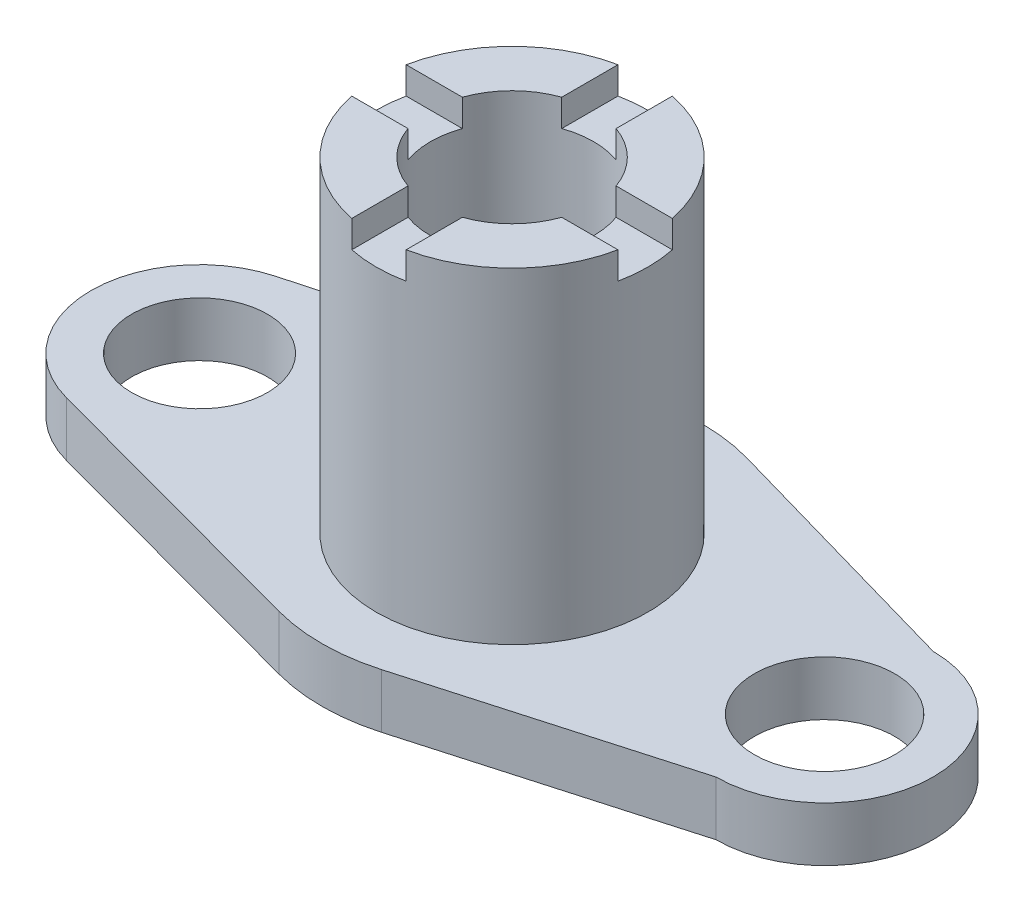
ISO-10303-21;
HEADER;
FILE_DESCRIPTION(('STEP AP214'),'2;1');
FILE_NAME('part.step','',(''),(''),'','','');
FILE_SCHEMA(('AUTOMOTIVE_DESIGN { 1 0 10303 214 1 1 1 1 }'));
ENDSEC;
DATA;
#1=APPLICATION_CONTEXT('core data for automotive mechanical design processes');
#2=APPLICATION_PROTOCOL_DEFINITION('international standard','automotive_design',2000,#1);
#3=PRODUCT_CONTEXT('',#1,'mechanical');
#4=PRODUCT('Part','Part','',(#3));
#5=PRODUCT_RELATED_PRODUCT_CATEGORY('part','',(#4));
#6=PRODUCT_DEFINITION_FORMATION('','',#4);
#7=PRODUCT_DEFINITION_CONTEXT('part definition',#1,'design');
#8=PRODUCT_DEFINITION('design','',#6,#7);
#9=PRODUCT_DEFINITION_SHAPE('','',#8);
#10=(LENGTH_UNIT() NAMED_UNIT(*) SI_UNIT(.MILLI.,.METRE.));
#11=(NAMED_UNIT(*) PLANE_ANGLE_UNIT() SI_UNIT($,.RADIAN.));
#12=(NAMED_UNIT(*) SI_UNIT($,.STERADIAN.) SOLID_ANGLE_UNIT());
#13=UNCERTAINTY_MEASURE_WITH_UNIT(LENGTH_MEASURE(1.E-05),#10,'distance_accuracy_value','');
#14=(GEOMETRIC_REPRESENTATION_CONTEXT(3) GLOBAL_UNCERTAINTY_ASSIGNED_CONTEXT((#13)) GLOBAL_UNIT_ASSIGNED_CONTEXT((#10,
#11,#12)) REPRESENTATION_CONTEXT('',''));
#15=CARTESIAN_POINT('',(0.,0.,0.));
#16=DIRECTION('',(0.,0.,1.));
#17=DIRECTION('',(1.,0.,0.));
#18=AXIS2_PLACEMENT_3D('',#15,#16,#17);
#19=CARTESIAN_POINT('',(0.,65.,0.));
#20=DIRECTION('',(0.,1.,0.));
#21=DIRECTION('',(0.,0.,1.));
#22=AXIS2_PLACEMENT_3D('',#19,#20,#21);
#23=PLANE('',#22);
#24=DIRECTION('',(0.,0.,-1.));
#25=VECTOR('',#24,1.);
#26=CARTESIAN_POINT('',(5.,65.,-25.0621356237309));
#27=LINE('',#26,#25);
#28=CARTESIAN_POINT('',(5.,65.,-14.1421356237309));
#29=VERTEX_POINT('',#28);
#30=CARTESIAN_POINT('',(5.,65.,-24.4948974278318));
#31=VERTEX_POINT('',#30);
#32=EDGE_CURVE('E249',#29,#31,#27,.T.);
#33=ORIENTED_EDGE('',*,*,#32,.F.);
#34=CARTESIAN_POINT('',(0.,65.,0.));
#35=DIRECTION('',(0.,1.,0.));
#36=DIRECTION('',(0.,0.,1.));
#37=AXIS2_PLACEMENT_3D('',#34,#35,#36);
#38=CIRCLE('',#37,15.);
#39=CARTESIAN_POINT('',(14.142135623731,65.,-4.99999999999995));
#40=VERTEX_POINT('',#39);
#41=EDGE_CURVE('E228',#40,#29,#38,.T.);
#42=ORIENTED_EDGE('',*,*,#41,.F.);
#43=DIRECTION('',(-1.,0.,0.));
#44=VECTOR('',#43,1.);
#45=CARTESIAN_POINT('',(25.062135623731,65.,-4.99999999999991));
#46=LINE('',#45,#44);
#47=CARTESIAN_POINT('',(24.4948974278318,65.,-4.99999999999991));
#48=VERTEX_POINT('',#47);
#49=EDGE_CURVE('E243',#48,#40,#46,.T.);
#50=ORIENTED_EDGE('',*,*,#49,.F.);
#51=CARTESIAN_POINT('',(0.,65.,0.));
#52=DIRECTION('',(0.,1.,0.));
#53=DIRECTION('',(0.,0.,1.));
#54=AXIS2_PLACEMENT_3D('',#51,#52,#53);
#55=CIRCLE('',#54,25.);
#56=EDGE_CURVE('E320',#48,#31,#55,.T.);
#57=ORIENTED_EDGE('',*,*,#56,.T.);
#58=EDGE_LOOP('',(#33,#42,#50,#57));
#59=FACE_BOUND('',#58,.T.);
#60=ADVANCED_FACE('F44',(#59),#23,.T.);
#61=DIRECTION('',(0.,0.,1.));
#62=VECTOR('',#61,1.);
#63=CARTESIAN_POINT('',(-4.99999999999999,65.,-25.0621356237309));
#64=LINE('',#63,#62);
#65=CARTESIAN_POINT('',(-4.99999999999999,65.,-24.4948974278318));
#66=VERTEX_POINT('',#65);
#67=CARTESIAN_POINT('',(-5.,65.,-14.1421356237309));
#68=VERTEX_POINT('',#67);
#69=EDGE_CURVE('E219',#66,#68,#64,.T.);
#70=ORIENTED_EDGE('',*,*,#69,.F.);
#71=CARTESIAN_POINT('',(-24.4948974278317,65.,-5.00000000000026));
#72=VERTEX_POINT('',#71);
#73=EDGE_CURVE('E416',#66,#72,#55,.T.);
#74=ORIENTED_EDGE('',*,*,#73,.T.);
#75=DIRECTION('',(-1.,0.,0.));
#76=VECTOR('',#75,1.);
#77=CARTESIAN_POINT('',(-25.0621356237309,65.,-5.00000000000027));
#78=LINE('',#77,#76);
#79=CARTESIAN_POINT('',(-14.1421356237309,65.,-5.00000000000015));
#80=VERTEX_POINT('',#79);
#81=EDGE_CURVE('E258',#80,#72,#78,.T.);
#82=ORIENTED_EDGE('',*,*,#81,.F.);
#83=EDGE_CURVE('E439',#68,#80,#38,.T.);
#84=ORIENTED_EDGE('',*,*,#83,.F.);
#85=EDGE_LOOP('',(#70,#74,#82,#84));
#86=FACE_BOUND('',#85,.T.);
#87=ADVANCED_FACE('F441',(#86),#23,.T.);
#88=DIRECTION('',(1.,0.,0.));
#89=VECTOR('',#88,1.);
#90=CARTESIAN_POINT('',(25.0621356237309,65.,5.00000000000009));
#91=LINE('',#90,#89);
#92=CARTESIAN_POINT('',(14.1421356237309,65.,5.00000000000005));
#93=VERTEX_POINT('',#92);
#94=CARTESIAN_POINT('',(24.4948974278318,65.,5.00000000000009));
#95=VERTEX_POINT('',#94);
#96=EDGE_CURVE('E241',#93,#95,#91,.T.);
#97=ORIENTED_EDGE('',*,*,#96,.F.);
#98=CARTESIAN_POINT('',(4.9999999999999,65.,14.142135623731));
#99=VERTEX_POINT('',#98);
#100=EDGE_CURVE('E310',#99,#93,#38,.T.);
#101=ORIENTED_EDGE('',*,*,#100,.F.);
#102=DIRECTION('',(0.,0.,-1.));
#103=VECTOR('',#102,1.);
#104=CARTESIAN_POINT('',(4.99999999999982,65.,25.062135623731));
#105=LINE('',#104,#103);
#106=CARTESIAN_POINT('',(4.99999999999982,65.,24.4948974278318));
#107=VERTEX_POINT('',#106);
#108=EDGE_CURVE('E260',#107,#99,#105,.T.);
#109=ORIENTED_EDGE('',*,*,#108,.F.);
#110=EDGE_CURVE('E311',#107,#95,#55,.T.);
#111=ORIENTED_EDGE('',*,*,#110,.T.);
#112=EDGE_LOOP('',(#97,#101,#109,#111));
#113=FACE_BOUND('',#112,.T.);
#114=ADVANCED_FACE('F406',(#113),#23,.T.);
#115=CARTESIAN_POINT('',(-57.5,5.,0.));
#116=DIRECTION('',(0.,1.,0.));
#117=DIRECTION('',(0.,0.,1.));
#118=AXIS2_PLACEMENT_3D('',#115,#116,#117);
#119=PLANE('',#118);
#120=CARTESIAN_POINT('',(0.,5.,0.));
#121=DIRECTION('',(0.,1.,0.));
#122=DIRECTION('',(0.,0.,1.));
#123=AXIS2_PLACEMENT_3D('',#120,#121,#122);
#124=CIRCLE('',#123,25.);
#125=CARTESIAN_POINT('',(0.,5.,25.));
#126=VERTEX_POINT('',#125);
#127=EDGE_CURVE('E315',#126,#126,#124,.T.);
#128=ORIENTED_EDGE('',*,*,#127,.F.);
#129=EDGE_LOOP('',(#128));
#130=FACE_BOUND('',#129,.T.);
#131=CARTESIAN_POINT('',(-57.5,5.,0.));
#132=DIRECTION('',(0.,1.,0.));
#133=DIRECTION('',(0.,0.,1.));
#134=AXIS2_PLACEMENT_3D('',#131,#132,#133);
#135=CIRCLE('',#134,12.5);
#136=CARTESIAN_POINT('',(-57.5,5.,12.5));
#137=VERTEX_POINT('',#136);
#138=EDGE_CURVE('E330',#137,#137,#135,.T.);
#139=ORIENTED_EDGE('',*,*,#138,.F.);
#140=EDGE_LOOP('',(#139));
#141=FACE_BOUND('',#140,.T.);
#142=CARTESIAN_POINT('',(-57.5,5.,0.));
#143=DIRECTION('',(0.,1.,0.));
#144=DIRECTION('',(0.,0.,1.));
#145=AXIS2_PLACEMENT_3D('',#142,#143,#144);
#146=CIRCLE('',#145,20.);
#147=CARTESIAN_POINT('',(-62.7173913043478,5.,-19.3074811401518));
#148=VERTEX_POINT('',#147);
#149=CARTESIAN_POINT('',(-62.7173913043478,5.,19.3074811401517));
#150=VERTEX_POINT('',#149);
#151=EDGE_CURVE('E334',#148,#150,#146,.T.);
#152=ORIENTED_EDGE('',*,*,#151,.T.);
#153=DIRECTION('',(0.965374057007588,0.,0.260869565217392));
#154=VECTOR('',#153,1.);
#155=CARTESIAN_POINT('',(-62.7173913043478,5.,19.3074811401517));
#156=LINE('',#155,#154);
#157=CARTESIAN_POINT('',(-9.13043478260871,5.,33.7880919952656));
#158=VERTEX_POINT('',#157);
#159=EDGE_CURVE('E338',#150,#158,#156,.T.);
#160=ORIENTED_EDGE('',*,*,#159,.T.);
#161=CARTESIAN_POINT('',(0.,5.,0.));
#162=DIRECTION('',(0.,1.,0.));
#163=DIRECTION('',(0.,0.,1.));
#164=AXIS2_PLACEMENT_3D('',#161,#162,#163);
#165=CIRCLE('',#164,35.);
#166=CARTESIAN_POINT('',(9.59703123668137,5.,33.6585351945411));
#167=VERTEX_POINT('',#166);
#168=EDGE_CURVE('E337',#158,#167,#165,.T.);
#169=ORIENTED_EDGE('',*,*,#168,.T.);
#170=DIRECTION('',(0.961672434129746,0.,-0.274200892476611));
#171=VECTOR('',#170,1.);
#172=CARTESIAN_POINT('',(9.59703123668137,5.,33.6585351945411));
#173=LINE('',#172,#171);
#174=CARTESIAN_POINT('',(57.5,5.,20.));
#175=VERTEX_POINT('',#174);
#176=EDGE_CURVE('E344',#167,#175,#173,.T.);
#177=ORIENTED_EDGE('',*,*,#176,.T.);
#178=CARTESIAN_POINT('',(57.5,5.,0.));
#179=DIRECTION('',(0.,1.,0.));
#180=DIRECTION('',(0.,0.,1.));
#181=AXIS2_PLACEMENT_3D('',#178,#179,#180);
#182=CIRCLE('',#181,20.);
#183=CARTESIAN_POINT('',(57.5,5.,-20.));
#184=VERTEX_POINT('',#183);
#185=EDGE_CURVE('E345',#175,#184,#182,.T.);
#186=ORIENTED_EDGE('',*,*,#185,.T.);
#187=DIRECTION('',(-0.961672434129746,0.,-0.274200892476611));
#188=VECTOR('',#187,1.);
#189=CARTESIAN_POINT('',(9.59703123668137,5.,-33.6585351945411));
#190=LINE('',#189,#188);
#191=CARTESIAN_POINT('',(9.59703123668136,5.,-33.6585351945411));
#192=VERTEX_POINT('',#191);
#193=EDGE_CURVE('E342',#184,#192,#190,.T.);
#194=ORIENTED_EDGE('',*,*,#193,.T.);
#195=CARTESIAN_POINT('',(0.,5.,0.));
#196=DIRECTION('',(0.,1.,0.));
#197=DIRECTION('',(0.,0.,1.));
#198=AXIS2_PLACEMENT_3D('',#195,#196,#197);
#199=CIRCLE('',#198,35.);
#200=CARTESIAN_POINT('',(-9.13043478260871,5.,-33.7880919952656));
#201=VERTEX_POINT('',#200);
#202=EDGE_CURVE('E350',#192,#201,#199,.T.);
#203=ORIENTED_EDGE('',*,*,#202,.T.);
#204=DIRECTION('',(-0.965374057007588,0.,0.260869565217391));
#205=VECTOR('',#204,1.);
#206=CARTESIAN_POINT('',(-62.7173913043478,5.,-19.3074811401518));
#207=LINE('',#206,#205);
#208=EDGE_CURVE('E349',#201,#148,#207,.T.);
#209=ORIENTED_EDGE('',*,*,#208,.T.);
#210=EDGE_LOOP('',(#152,#160,#169,#177,#186,#194,#203,#209));
#211=FACE_BOUND('',#210,.T.);
#212=CARTESIAN_POINT('',(57.5,5.,0.));
#213=DIRECTION('',(0.,1.,0.));
#214=DIRECTION('',(0.,0.,1.));
#215=AXIS2_PLACEMENT_3D('',#212,#213,#214);
#216=CIRCLE('',#215,12.9208356415336);
#217=CARTESIAN_POINT('',(57.5,5.,12.9208356415336));
#218=VERTEX_POINT('',#217);
#219=EDGE_CURVE('E321',#218,#218,#216,.T.);
#220=ORIENTED_EDGE('',*,*,#219,.F.);
#221=EDGE_LOOP('',(#220));
#222=FACE_BOUND('',#221,.T.);
#223=ADVANCED_FACE('F462',(#130,#141,#211,#222),#119,.T.);
#224=CARTESIAN_POINT('',(-57.5,-5.,0.));
#225=DIRECTION('',(0.,1.,0.));
#226=DIRECTION('',(0.,0.,1.));
#227=AXIS2_PLACEMENT_3D('',#224,#225,#226);
#228=PLANE('',#227);
#229=CARTESIAN_POINT('',(-57.5,-5.,0.));
#230=DIRECTION('',(0.,1.,0.));
#231=DIRECTION('',(0.,0.,1.));
#232=AXIS2_PLACEMENT_3D('',#229,#230,#231);
#233=CIRCLE('',#232,20.);
#234=CARTESIAN_POINT('',(-62.7173913043478,-5.,-19.3074811401518));
#235=VERTEX_POINT('',#234);
#236=CARTESIAN_POINT('',(-62.7173913043478,-5.,19.3074811401517));
#237=VERTEX_POINT('',#236);
#238=EDGE_CURVE('E329',#235,#237,#233,.T.);
#239=ORIENTED_EDGE('',*,*,#238,.F.);
#240=DIRECTION('',(-0.965374057007588,0.,0.260869565217391));
#241=VECTOR('',#240,1.);
#242=CARTESIAN_POINT('',(-62.7173913043478,-5.,-19.3074811401518));
#243=LINE('',#242,#241);
#244=CARTESIAN_POINT('',(-9.13043478260871,-5.,-33.7880919952656));
#245=VERTEX_POINT('',#244);
#246=EDGE_CURVE('E340',#245,#235,#243,.T.);
#247=ORIENTED_EDGE('',*,*,#246,.F.);
#248=CARTESIAN_POINT('',(0.,-5.,0.));
#249=DIRECTION('',(0.,1.,0.));
#250=DIRECTION('',(0.,0.,1.));
#251=AXIS2_PLACEMENT_3D('',#248,#249,#250);
#252=CIRCLE('',#251,35.);
#253=CARTESIAN_POINT('',(9.59703123668136,-5.,-33.6585351945411));
#254=VERTEX_POINT('',#253);
#255=EDGE_CURVE('E365',#254,#245,#252,.T.);
#256=ORIENTED_EDGE('',*,*,#255,.F.);
#257=DIRECTION('',(-0.961672434129746,0.,-0.274200892476611));
#258=VECTOR('',#257,1.);
#259=CARTESIAN_POINT('',(9.59703123668137,-5.,-33.6585351945411));
#260=LINE('',#259,#258);
#261=CARTESIAN_POINT('',(57.5,-5.,-20.));
#262=VERTEX_POINT('',#261);
#263=EDGE_CURVE('E362',#262,#254,#260,.T.);
#264=ORIENTED_EDGE('',*,*,#263,.F.);
#265=CARTESIAN_POINT('',(57.5,-5.,0.));
#266=DIRECTION('',(0.,1.,0.));
#267=DIRECTION('',(0.,0.,1.));
#268=AXIS2_PLACEMENT_3D('',#265,#266,#267);
#269=CIRCLE('',#268,20.);
#270=CARTESIAN_POINT('',(57.5,-5.,20.));
#271=VERTEX_POINT('',#270);
#272=EDGE_CURVE('E357',#271,#262,#269,.T.);
#273=ORIENTED_EDGE('',*,*,#272,.F.);
#274=DIRECTION('',(0.961672434129746,0.,-0.274200892476611));
#275=VECTOR('',#274,1.);
#276=CARTESIAN_POINT('',(9.59703123668137,-5.,33.6585351945411));
#277=LINE('',#276,#275);
#278=CARTESIAN_POINT('',(9.59703123668137,-5.,33.6585351945411));
#279=VERTEX_POINT('',#278);
#280=EDGE_CURVE('E360',#279,#271,#277,.T.);
#281=ORIENTED_EDGE('',*,*,#280,.F.);
#282=CARTESIAN_POINT('',(0.,-5.,0.));
#283=DIRECTION('',(0.,1.,0.));
#284=DIRECTION('',(0.,0.,1.));
#285=AXIS2_PLACEMENT_3D('',#282,#283,#284);
#286=CIRCLE('',#285,35.);
#287=CARTESIAN_POINT('',(-9.13043478260871,-5.,33.7880919952656));
#288=VERTEX_POINT('',#287);
#289=EDGE_CURVE('E359',#288,#279,#286,.T.);
#290=ORIENTED_EDGE('',*,*,#289,.F.);
#291=DIRECTION('',(0.965374057007588,0.,0.260869565217392));
#292=VECTOR('',#291,1.);
#293=CARTESIAN_POINT('',(-62.7173913043478,-5.,19.3074811401517));
#294=LINE('',#293,#292);
#295=EDGE_CURVE('E352',#237,#288,#294,.T.);
#296=ORIENTED_EDGE('',*,*,#295,.F.);
#297=EDGE_LOOP('',(#239,#247,#256,#264,#273,#281,#290,#296));
#298=FACE_BOUND('',#297,.T.);
#299=CARTESIAN_POINT('',(-57.5,-5.,0.));
#300=DIRECTION('',(0.,1.,0.));
#301=DIRECTION('',(0.,0.,1.));
#302=AXIS2_PLACEMENT_3D('',#299,#300,#301);
#303=CIRCLE('',#302,12.5);
#304=CARTESIAN_POINT('',(-57.5,-5.,12.5));
#305=VERTEX_POINT('',#304);
#306=EDGE_CURVE('E322',#305,#305,#303,.T.);
#307=ORIENTED_EDGE('',*,*,#306,.T.);
#308=EDGE_LOOP('',(#307));
#309=FACE_BOUND('',#308,.T.);
#310=CARTESIAN_POINT('',(57.5,-5.,0.));
#311=DIRECTION('',(0.,1.,0.));
#312=DIRECTION('',(0.,0.,1.));
#313=AXIS2_PLACEMENT_3D('',#310,#311,#312);
#314=CIRCLE('',#313,12.9208356415336);
#315=CARTESIAN_POINT('',(57.5,-5.,12.9208356415336));
#316=VERTEX_POINT('',#315);
#317=EDGE_CURVE('E316',#316,#316,#314,.T.);
#318=ORIENTED_EDGE('',*,*,#317,.T.);
#319=EDGE_LOOP('',(#318));
#320=FACE_BOUND('',#319,.T.);
#321=ADVANCED_FACE('F486',(#298,#309,#320),#228,.F.);
#322=CARTESIAN_POINT('',(-57.5,5.,0.));
#323=DIRECTION('',(0.,-1.,0.));
#324=DIRECTION('',(0.,0.,-1.));
#325=AXIS2_PLACEMENT_3D('',#322,#323,#324);
#326=CYLINDRICAL_SURFACE('',#325,20.);
#327=ORIENTED_EDGE('',*,*,#238,.T.);
#328=DIRECTION('',(0.,-1.,0.));
#329=VECTOR('',#328,1.);
#330=CARTESIAN_POINT('',(-62.7173913043478,5.,19.3074811401517));
#331=LINE('',#330,#329);
#332=EDGE_CURVE('E390',#150,#237,#331,.T.);
#333=ORIENTED_EDGE('',*,*,#332,.F.);
#334=ORIENTED_EDGE('',*,*,#151,.F.);
#335=DIRECTION('',(0.,-1.,0.));
#336=VECTOR('',#335,1.);
#337=CARTESIAN_POINT('',(-62.7173913043478,5.,-19.3074811401518));
#338=LINE('',#337,#336);
#339=EDGE_CURVE('E353',#148,#235,#338,.T.);
#340=ORIENTED_EDGE('',*,*,#339,.T.);
#341=EDGE_LOOP('',(#327,#333,#334,#340));
#342=FACE_BOUND('',#341,.T.);
#343=ADVANCED_FACE('F50',(#342),#326,.T.);
#344=CARTESIAN_POINT('',(-62.7173913043478,5.,19.3074811401517));
#345=DIRECTION('',(0.260869565217392,0.,-0.965374057007588));
#346=DIRECTION('',(-0.965374057007588,0.,-0.260869565217392));
#347=AXIS2_PLACEMENT_3D('',#344,#345,#346);
#348=PLANE('',#347);
#349=ORIENTED_EDGE('',*,*,#295,.T.);
#350=DIRECTION('',(0.,-1.,0.));
#351=VECTOR('',#350,1.);
#352=CARTESIAN_POINT('',(-9.13043478260871,5.,33.7880919952656));
#353=LINE('',#352,#351);
#354=EDGE_CURVE('E383',#158,#288,#353,.T.);
#355=ORIENTED_EDGE('',*,*,#354,.F.);
#356=ORIENTED_EDGE('',*,*,#159,.F.);
#357=ORIENTED_EDGE('',*,*,#332,.T.);
#358=EDGE_LOOP('',(#349,#355,#356,#357));
#359=FACE_BOUND('',#358,.T.);
#360=ADVANCED_FACE('F517',(#359),#348,.F.);
#361=CARTESIAN_POINT('',(0.,5.,0.));
#362=DIRECTION('',(0.,-1.,0.));
#363=DIRECTION('',(0.,0.,-1.));
#364=AXIS2_PLACEMENT_3D('',#361,#362,#363);
#365=CYLINDRICAL_SURFACE('',#364,35.);
#366=ORIENTED_EDGE('',*,*,#289,.T.);
#367=DIRECTION('',(0.,-1.,0.));
#368=VECTOR('',#367,1.);
#369=CARTESIAN_POINT('',(9.59703123668137,5.,33.6585351945411));
#370=LINE('',#369,#368);
#371=EDGE_CURVE('E381',#167,#279,#370,.T.);
#372=ORIENTED_EDGE('',*,*,#371,.F.);
#373=ORIENTED_EDGE('',*,*,#168,.F.);
#374=ORIENTED_EDGE('',*,*,#354,.T.);
#375=EDGE_LOOP('',(#366,#372,#373,#374));
#376=FACE_BOUND('',#375,.T.);
#377=ADVANCED_FACE('F518',(#376),#365,.T.);
#378=CARTESIAN_POINT('',(9.59703123668137,5.,33.6585351945411));
#379=DIRECTION('',(-0.274200892476611,0.,-0.961672434129746));
#380=DIRECTION('',(-0.961672434129746,0.,0.274200892476611));
#381=AXIS2_PLACEMENT_3D('',#378,#379,#380);
#382=PLANE('',#381);
#383=ORIENTED_EDGE('',*,*,#280,.T.);
#384=DIRECTION('',(0.,-1.,0.));
#385=VECTOR('',#384,1.);
#386=CARTESIAN_POINT('',(57.5,5.,20.));
#387=LINE('',#386,#385);
#388=EDGE_CURVE('E378',#175,#271,#387,.T.);
#389=ORIENTED_EDGE('',*,*,#388,.F.);
#390=ORIENTED_EDGE('',*,*,#176,.F.);
#391=ORIENTED_EDGE('',*,*,#371,.T.);
#392=EDGE_LOOP('',(#383,#389,#390,#391));
#393=FACE_BOUND('',#392,.T.);
#394=ADVANCED_FACE('F515',(#393),#382,.F.);
#395=CARTESIAN_POINT('',(57.5,5.,0.));
#396=DIRECTION('',(0.,-1.,0.));
#397=DIRECTION('',(0.,0.,-1.));
#398=AXIS2_PLACEMENT_3D('',#395,#396,#397);
#399=CYLINDRICAL_SURFACE('',#398,20.);
#400=ORIENTED_EDGE('',*,*,#272,.T.);
#401=DIRECTION('',(0.,-1.,0.));
#402=VECTOR('',#401,1.);
#403=CARTESIAN_POINT('',(57.5,5.,-20.));
#404=LINE('',#403,#402);
#405=EDGE_CURVE('E374',#184,#262,#404,.T.);
#406=ORIENTED_EDGE('',*,*,#405,.F.);
#407=ORIENTED_EDGE('',*,*,#185,.F.);
#408=ORIENTED_EDGE('',*,*,#388,.T.);
#409=EDGE_LOOP('',(#400,#406,#407,#408));
#410=FACE_BOUND('',#409,.T.);
#411=ADVANCED_FACE('F510',(#410),#399,.T.);
#412=CARTESIAN_POINT('',(9.59703123668137,5.,-33.6585351945411));
#413=DIRECTION('',(-0.274200892476611,0.,0.961672434129746));
#414=DIRECTION('',(0.961672434129746,0.,0.274200892476611));
#415=AXIS2_PLACEMENT_3D('',#412,#413,#414);
#416=PLANE('',#415);
#417=ORIENTED_EDGE('',*,*,#263,.T.);
#418=DIRECTION('',(0.,-1.,0.));
#419=VECTOR('',#418,1.);
#420=CARTESIAN_POINT('',(9.59703123668136,5.,-33.6585351945411));
#421=LINE('',#420,#419);
#422=EDGE_CURVE('E375',#192,#254,#421,.T.);
#423=ORIENTED_EDGE('',*,*,#422,.F.);
#424=ORIENTED_EDGE('',*,*,#193,.F.);
#425=ORIENTED_EDGE('',*,*,#405,.T.);
#426=EDGE_LOOP('',(#417,#423,#424,#425));
#427=FACE_BOUND('',#426,.T.);
#428=ADVANCED_FACE('F502',(#427),#416,.F.);
#429=CARTESIAN_POINT('',(0.,5.,0.));
#430=DIRECTION('',(0.,-1.,0.));
#431=DIRECTION('',(0.,0.,-1.));
#432=AXIS2_PLACEMENT_3D('',#429,#430,#431);
#433=CYLINDRICAL_SURFACE('',#432,35.);
#434=ORIENTED_EDGE('',*,*,#255,.T.);
#435=DIRECTION('',(0.,-1.,0.));
#436=VECTOR('',#435,1.);
#437=CARTESIAN_POINT('',(-9.13043478260871,5.,-33.7880919952656));
#438=LINE('',#437,#436);
#439=EDGE_CURVE('E369',#201,#245,#438,.T.);
#440=ORIENTED_EDGE('',*,*,#439,.F.);
#441=ORIENTED_EDGE('',*,*,#202,.F.);
#442=ORIENTED_EDGE('',*,*,#422,.T.);
#443=EDGE_LOOP('',(#434,#440,#441,#442));
#444=FACE_BOUND('',#443,.T.);
#445=ADVANCED_FACE('F498',(#444),#433,.T.);
#446=CARTESIAN_POINT('',(-62.7173913043478,5.,-19.3074811401518));
#447=DIRECTION('',(0.260869565217391,0.,0.965374057007588));
#448=DIRECTION('',(0.965374057007588,0.,-0.260869565217391));
#449=AXIS2_PLACEMENT_3D('',#446,#447,#448);
#450=PLANE('',#449);
#451=ORIENTED_EDGE('',*,*,#246,.T.);
#452=ORIENTED_EDGE('',*,*,#339,.F.);
#453=ORIENTED_EDGE('',*,*,#208,.F.);
#454=ORIENTED_EDGE('',*,*,#439,.T.);
#455=EDGE_LOOP('',(#451,#452,#453,#454));
#456=FACE_BOUND('',#455,.T.);
#457=ADVANCED_FACE('F500',(#456),#450,.F.);
#458=CARTESIAN_POINT('',(-57.5,5.,0.));
#459=DIRECTION('',(0.,-1.,0.));
#460=DIRECTION('',(0.,0.,-1.));
#461=AXIS2_PLACEMENT_3D('',#458,#459,#460);
#462=CYLINDRICAL_SURFACE('',#461,12.5);
#463=ORIENTED_EDGE('',*,*,#138,.T.);
#464=EDGE_LOOP('',(#463));
#465=FACE_BOUND('',#464,.T.);
#466=ORIENTED_EDGE('',*,*,#306,.F.);
#467=EDGE_LOOP('',(#466));
#468=FACE_BOUND('',#467,.T.);
#469=ADVANCED_FACE('F477',(#465,#468),#462,.F.);
#470=CARTESIAN_POINT('',(57.5,5.,0.));
#471=DIRECTION('',(0.,-1.,0.));
#472=DIRECTION('',(0.,0.,-1.));
#473=AXIS2_PLACEMENT_3D('',#470,#471,#472);
#474=CYLINDRICAL_SURFACE('',#473,12.9208356415336);
#475=ORIENTED_EDGE('',*,*,#219,.T.);
#476=EDGE_LOOP('',(#475));
#477=FACE_BOUND('',#476,.T.);
#478=ORIENTED_EDGE('',*,*,#317,.F.);
#479=EDGE_LOOP('',(#478));
#480=FACE_BOUND('',#479,.T.);
#481=ADVANCED_FACE('F475',(#477,#480),#474,.F.);
#482=DIRECTION('',(0.,0.,1.));
#483=VECTOR('',#482,1.);
#484=CARTESIAN_POINT('',(-5.00000000000018,65.,25.0621356237309));
#485=LINE('',#484,#483);
#486=CARTESIAN_POINT('',(-5.0000000000001,65.,14.1421356237309));
#487=VERTEX_POINT('',#486);
#488=CARTESIAN_POINT('',(-5.00000000000017,65.,24.4948974278317));
#489=VERTEX_POINT('',#488);
#490=EDGE_CURVE('E238',#487,#489,#485,.T.);
#491=ORIENTED_EDGE('',*,*,#490,.F.);
#492=CARTESIAN_POINT('',(-14.142135623731,65.,4.99999999999985));
#493=VERTEX_POINT('',#492);
#494=EDGE_CURVE('E306',#493,#487,#38,.T.);
#495=ORIENTED_EDGE('',*,*,#494,.F.);
#496=DIRECTION('',(1.,0.,0.));
#497=VECTOR('',#496,1.);
#498=CARTESIAN_POINT('',(-25.062135623731,65.,4.99999999999973));
#499=LINE('',#498,#497);
#500=CARTESIAN_POINT('',(-24.4948974278318,65.,4.99999999999974));
#501=VERTEX_POINT('',#500);
#502=EDGE_CURVE('E271',#501,#493,#499,.T.);
#503=ORIENTED_EDGE('',*,*,#502,.F.);
#504=EDGE_CURVE('E318',#501,#489,#55,.T.);
#505=ORIENTED_EDGE('',*,*,#504,.T.);
#506=EDGE_LOOP('',(#491,#495,#503,#505));
#507=FACE_BOUND('',#506,.T.);
#508=ADVANCED_FACE('F427',(#507),#23,.T.);
#509=CARTESIAN_POINT('',(0.,65.,0.));
#510=DIRECTION('',(0.,-1.,0.));
#511=DIRECTION('',(0.,0.,-1.));
#512=AXIS2_PLACEMENT_3D('',#509,#510,#511);
#513=CYLINDRICAL_SURFACE('',#512,25.);
#514=CARTESIAN_POINT('',(0.,60.,0.));
#515=DIRECTION('',(0.,1.,0.));
#516=DIRECTION('',(0.,0.,1.));
#517=AXIS2_PLACEMENT_3D('',#514,#515,#516);
#518=CIRCLE('',#517,25.);
#519=CARTESIAN_POINT('',(5.,60.,-24.4948974278318));
#520=VERTEX_POINT('',#519);
#521=CARTESIAN_POINT('',(-4.99999999999999,60.,-24.4948974278318));
#522=VERTEX_POINT('',#521);
#523=EDGE_CURVE('E301',#520,#522,#518,.T.);
#524=ORIENTED_EDGE('',*,*,#523,.F.);
#525=DIRECTION('',(0.,-1.,0.));
#526=VECTOR('',#525,1.);
#527=CARTESIAN_POINT('',(5.,65.,-24.4948974278318));
#528=LINE('',#527,#526);
#529=EDGE_CURVE('E218',#520,#31,#528,.F.);
#530=ORIENTED_EDGE('',*,*,#529,.T.);
#531=ORIENTED_EDGE('',*,*,#56,.F.);
#532=DIRECTION('',(0.,-1.,0.));
#533=VECTOR('',#532,1.);
#534=CARTESIAN_POINT('',(24.4948974278318,65.,-4.99999999999991));
#535=LINE('',#534,#533);
#536=CARTESIAN_POINT('',(24.4948974278318,60.,-4.99999999999991));
#537=VERTEX_POINT('',#536);
#538=EDGE_CURVE('E297',#48,#537,#535,.T.);
#539=ORIENTED_EDGE('',*,*,#538,.T.);
#540=CARTESIAN_POINT('',(0.,60.,0.));
#541=DIRECTION('',(0.,-1.,0.));
#542=DIRECTION('',(0.,0.,-1.));
#543=AXIS2_PLACEMENT_3D('',#540,#541,#542);
#544=CIRCLE('',#543,25.);
#545=CARTESIAN_POINT('',(24.4948974278318,60.,5.00000000000009));
#546=VERTEX_POINT('',#545);
#547=EDGE_CURVE('E291',#537,#546,#544,.T.);
#548=ORIENTED_EDGE('',*,*,#547,.T.);
#549=DIRECTION('',(0.,-1.,0.));
#550=VECTOR('',#549,1.);
#551=CARTESIAN_POINT('',(24.4948974278318,65.,5.00000000000009));
#552=LINE('',#551,#550);
#553=EDGE_CURVE('E298',#546,#95,#552,.F.);
#554=ORIENTED_EDGE('',*,*,#553,.T.);
#555=ORIENTED_EDGE('',*,*,#110,.F.);
#556=DIRECTION('',(0.,-1.,0.));
#557=VECTOR('',#556,1.);
#558=CARTESIAN_POINT('',(4.99999999999982,65.,24.4948974278318));
#559=LINE('',#558,#557);
#560=CARTESIAN_POINT('',(4.99999999999982,60.,24.4948974278318));
#561=VERTEX_POINT('',#560);
#562=EDGE_CURVE('E287',#107,#561,#559,.T.);
#563=ORIENTED_EDGE('',*,*,#562,.T.);
#564=CARTESIAN_POINT('',(0.,60.,0.));
#565=DIRECTION('',(0.,-1.,0.));
#566=DIRECTION('',(0.,0.,-1.));
#567=AXIS2_PLACEMENT_3D('',#564,#565,#566);
#568=CIRCLE('',#567,25.);
#569=CARTESIAN_POINT('',(-5.00000000000017,60.,24.4948974278317));
#570=VERTEX_POINT('',#569);
#571=EDGE_CURVE('E282',#561,#570,#568,.T.);
#572=ORIENTED_EDGE('',*,*,#571,.T.);
#573=DIRECTION('',(0.,-1.,0.));
#574=VECTOR('',#573,1.);
#575=CARTESIAN_POINT('',(-5.00000000000017,65.,24.4948974278317));
#576=LINE('',#575,#574);
#577=EDGE_CURVE('E286',#570,#489,#576,.F.);
#578=ORIENTED_EDGE('',*,*,#577,.T.);
#579=ORIENTED_EDGE('',*,*,#504,.F.);
#580=DIRECTION('',(0.,-1.,0.));
#581=VECTOR('',#580,1.);
#582=CARTESIAN_POINT('',(-24.4948974278318,65.,4.99999999999974));
#583=LINE('',#582,#581);
#584=CARTESIAN_POINT('',(-24.4948974278318,60.,4.99999999999974));
#585=VERTEX_POINT('',#584);
#586=EDGE_CURVE('E283',#501,#585,#583,.T.);
#587=ORIENTED_EDGE('',*,*,#586,.T.);
#588=CARTESIAN_POINT('',(0.,60.,0.));
#589=DIRECTION('',(0.,-1.,0.));
#590=DIRECTION('',(0.,0.,-1.));
#591=AXIS2_PLACEMENT_3D('',#588,#589,#590);
#592=CIRCLE('',#591,25.);
#593=CARTESIAN_POINT('',(-24.4948974278317,60.,-5.00000000000026));
#594=VERTEX_POINT('',#593);
#595=EDGE_CURVE('E230',#585,#594,#592,.T.);
#596=ORIENTED_EDGE('',*,*,#595,.T.);
#597=DIRECTION('',(0.,-1.,0.));
#598=VECTOR('',#597,1.);
#599=CARTESIAN_POINT('',(-24.4948974278317,65.,-5.00000000000026));
#600=LINE('',#599,#598);
#601=EDGE_CURVE('E229',#594,#72,#600,.F.);
#602=ORIENTED_EDGE('',*,*,#601,.T.);
#603=ORIENTED_EDGE('',*,*,#73,.F.);
#604=DIRECTION('',(0.,-1.,0.));
#605=VECTOR('',#604,1.);
#606=CARTESIAN_POINT('',(-4.99999999999999,65.,-24.4948974278318));
#607=LINE('',#606,#605);
#608=EDGE_CURVE('E303',#66,#522,#607,.T.);
#609=ORIENTED_EDGE('',*,*,#608,.T.);
#610=EDGE_LOOP('',(#524,#530,#531,#539,#548,#554,#555,#563,#572,#578,#579,#587,#596,#602,#603,#609));
#611=FACE_BOUND('',#610,.T.);
#612=ORIENTED_EDGE('',*,*,#127,.T.);
#613=EDGE_LOOP('',(#612));
#614=FACE_BOUND('',#613,.T.);
#615=ADVANCED_FACE('F414',(#611,#614),#513,.T.);
#616=CARTESIAN_POINT('',(0.,65.,0.));
#617=DIRECTION('',(0.,-1.,0.));
#618=DIRECTION('',(0.,0.,-1.));
#619=AXIS2_PLACEMENT_3D('',#616,#617,#618);
#620=CYLINDRICAL_SURFACE('',#619,15.);
#621=DIRECTION('',(0.,1.,0.));
#622=VECTOR('',#621,1.);
#623=CARTESIAN_POINT('',(5.,60.,-14.1421356237309));
#624=LINE('',#623,#622);
#625=CARTESIAN_POINT('',(5.,60.,-14.1421356237309));
#626=VERTEX_POINT('',#625);
#627=EDGE_CURVE('E216',#626,#29,#624,.T.);
#628=ORIENTED_EDGE('',*,*,#627,.F.);
#629=CARTESIAN_POINT('',(0.,60.,0.));
#630=DIRECTION('',(0.,1.,0.));
#631=DIRECTION('',(0.,0.,1.));
#632=AXIS2_PLACEMENT_3D('',#629,#630,#631);
#633=CIRCLE('',#632,15.);
#634=CARTESIAN_POINT('',(-5.,60.,-14.142135623731));
#635=VERTEX_POINT('',#634);
#636=EDGE_CURVE('E12',#626,#635,#633,.T.);
#637=ORIENTED_EDGE('',*,*,#636,.T.);
#638=DIRECTION('',(0.,1.,0.));
#639=VECTOR('',#638,1.);
#640=CARTESIAN_POINT('',(-5.,60.,-14.1421356237309));
#641=LINE('',#640,#639);
#642=EDGE_CURVE('E58',#635,#68,#641,.T.);
#643=ORIENTED_EDGE('',*,*,#642,.T.);
#644=ORIENTED_EDGE('',*,*,#83,.T.);
#645=DIRECTION('',(0.,1.,0.));
#646=VECTOR('',#645,1.);
#647=CARTESIAN_POINT('',(-14.1421356237309,60.,-5.00000000000015));
#648=LINE('',#647,#646);
#649=CARTESIAN_POINT('',(-14.1421356237309,60.,-5.00000000000015));
#650=VERTEX_POINT('',#649);
#651=EDGE_CURVE('E264',#650,#80,#648,.T.);
#652=ORIENTED_EDGE('',*,*,#651,.F.);
#653=CARTESIAN_POINT('',(0.,60.,0.));
#654=DIRECTION('',(0.,-1.,0.));
#655=DIRECTION('',(0.,0.,-1.));
#656=AXIS2_PLACEMENT_3D('',#653,#654,#655);
#657=CIRCLE('',#656,15.);
#658=CARTESIAN_POINT('',(-14.142135623731,60.,4.99999999999985));
#659=VERTEX_POINT('',#658);
#660=EDGE_CURVE('E391',#659,#650,#657,.T.);
#661=ORIENTED_EDGE('',*,*,#660,.F.);
#662=DIRECTION('',(0.,1.,0.));
#663=VECTOR('',#662,1.);
#664=CARTESIAN_POINT('',(-14.142135623731,60.,4.99999999999985));
#665=LINE('',#664,#663);
#666=EDGE_CURVE('E268',#659,#493,#665,.T.);
#667=ORIENTED_EDGE('',*,*,#666,.T.);
#668=ORIENTED_EDGE('',*,*,#494,.T.);
#669=DIRECTION('',(0.,1.,0.));
#670=VECTOR('',#669,1.);
#671=CARTESIAN_POINT('',(-5.0000000000001,60.,14.1421356237309));
#672=LINE('',#671,#670);
#673=CARTESIAN_POINT('',(-5.0000000000001,60.,14.1421356237309));
#674=VERTEX_POINT('',#673);
#675=EDGE_CURVE('E247',#674,#487,#672,.T.);
#676=ORIENTED_EDGE('',*,*,#675,.F.);
#677=CARTESIAN_POINT('',(0.,60.,0.));
#678=DIRECTION('',(0.,-1.,0.));
#679=DIRECTION('',(0.,0.,-1.));
#680=AXIS2_PLACEMENT_3D('',#677,#678,#679);
#681=CIRCLE('',#680,15.);
#682=CARTESIAN_POINT('',(4.9999999999999,60.,14.142135623731));
#683=VERTEX_POINT('',#682);
#684=EDGE_CURVE('E394',#683,#674,#681,.T.);
#685=ORIENTED_EDGE('',*,*,#684,.F.);
#686=DIRECTION('',(0.,1.,0.));
#687=VECTOR('',#686,1.);
#688=CARTESIAN_POINT('',(4.9999999999999,60.,14.142135623731));
#689=LINE('',#688,#687);
#690=EDGE_CURVE('E251',#683,#99,#689,.T.);
#691=ORIENTED_EDGE('',*,*,#690,.T.);
#692=ORIENTED_EDGE('',*,*,#100,.T.);
#693=DIRECTION('',(0.,1.,0.));
#694=VECTOR('',#693,1.);
#695=CARTESIAN_POINT('',(14.1421356237309,60.,5.00000000000005));
#696=LINE('',#695,#694);
#697=CARTESIAN_POINT('',(14.1421356237309,60.,5.00000000000005));
#698=VERTEX_POINT('',#697);
#699=EDGE_CURVE('E237',#698,#93,#696,.T.);
#700=ORIENTED_EDGE('',*,*,#699,.F.);
#701=CARTESIAN_POINT('',(0.,60.,0.));
#702=DIRECTION('',(0.,-1.,0.));
#703=DIRECTION('',(0.,0.,-1.));
#704=AXIS2_PLACEMENT_3D('',#701,#702,#703);
#705=CIRCLE('',#704,15.);
#706=CARTESIAN_POINT('',(14.142135623731,60.,-4.99999999999995));
#707=VERTEX_POINT('',#706);
#708=EDGE_CURVE('E52',#707,#698,#705,.T.);
#709=ORIENTED_EDGE('',*,*,#708,.F.);
#710=DIRECTION('',(0.,1.,0.));
#711=VECTOR('',#710,1.);
#712=CARTESIAN_POINT('',(14.142135623731,60.,-4.99999999999995));
#713=LINE('',#712,#711);
#714=EDGE_CURVE('E70',#707,#40,#713,.T.);
#715=ORIENTED_EDGE('',*,*,#714,.T.);
#716=ORIENTED_EDGE('',*,*,#41,.T.);
#717=EDGE_LOOP('',(#628,#637,#643,#644,#652,#661,#667,#668,#676,#685,#691,#692,#700,#709,#715,#716));
#718=FACE_BOUND('',#717,.T.);
#719=CARTESIAN_POINT('',(0.,5.,0.));
#720=DIRECTION('',(0.,1.,0.));
#721=DIRECTION('',(0.,0.,1.));
#722=AXIS2_PLACEMENT_3D('',#719,#720,#721);
#723=CIRCLE('',#722,15.);
#724=CARTESIAN_POINT('',(0.,5.,15.));
#725=VERTEX_POINT('',#724);
#726=EDGE_CURVE('E388',#725,#725,#723,.F.);
#727=ORIENTED_EDGE('',*,*,#726,.T.);
#728=EDGE_LOOP('',(#727));
#729=FACE_BOUND('',#728,.T.);
#730=ADVANCED_FACE('F224',(#718,#729),#620,.F.);
#731=ORIENTED_EDGE('',*,*,#726,.F.);
#732=EDGE_LOOP('',(#731));
#733=FACE_BOUND('',#732,.T.);
#734=ADVANCED_FACE('F453',(#733),#119,.T.);
#735=CARTESIAN_POINT('',(-25.062135623731,60.,4.99999999999973));
#736=DIRECTION('',(0.,0.,1.));
#737=DIRECTION('',(1.,0.,0.));
#738=AXIS2_PLACEMENT_3D('',#735,#736,#737);
#739=PLANE('',#738);
#740=ORIENTED_EDGE('',*,*,#502,.T.);
#741=ORIENTED_EDGE('',*,*,#666,.F.);
#742=DIRECTION('',(1.,0.,0.));
#743=VECTOR('',#742,1.);
#744=CARTESIAN_POINT('',(-25.062135623731,60.,4.99999999999973));
#745=LINE('',#744,#743);
#746=EDGE_CURVE('E270',#585,#659,#745,.T.);
#747=ORIENTED_EDGE('',*,*,#746,.F.);
#748=ORIENTED_EDGE('',*,*,#586,.F.);
#749=EDGE_LOOP('',(#740,#741,#747,#748));
#750=FACE_BOUND('',#749,.T.);
#751=ADVANCED_FACE('F451',(#750),#739,.F.);
#752=CARTESIAN_POINT('',(-25.0621356237309,60.,-5.00000000000027));
#753=DIRECTION('',(0.,0.,-1.));
#754=DIRECTION('',(-1.,0.,0.));
#755=AXIS2_PLACEMENT_3D('',#752,#753,#754);
#756=PLANE('',#755);
#757=DIRECTION('',(-1.,0.,0.));
#758=VECTOR('',#757,1.);
#759=CARTESIAN_POINT('',(-25.0621356237309,60.,-5.00000000000027));
#760=LINE('',#759,#758);
#761=EDGE_CURVE('E272',#650,#594,#760,.T.);
#762=ORIENTED_EDGE('',*,*,#761,.F.);
#763=ORIENTED_EDGE('',*,*,#651,.T.);
#764=ORIENTED_EDGE('',*,*,#81,.T.);
#765=ORIENTED_EDGE('',*,*,#601,.F.);
#766=EDGE_LOOP('',(#762,#763,#764,#765));
#767=FACE_BOUND('',#766,.T.);
#768=ADVANCED_FACE('F450',(#767),#756,.F.);
#769=CARTESIAN_POINT('',(0.,60.,0.));
#770=DIRECTION('',(0.,-1.,0.));
#771=DIRECTION('',(0.,0.,-1.));
#772=AXIS2_PLACEMENT_3D('',#769,#770,#771);
#773=PLANE('',#772);
#774=ORIENTED_EDGE('',*,*,#746,.T.);
#775=ORIENTED_EDGE('',*,*,#660,.T.);
#776=ORIENTED_EDGE('',*,*,#761,.T.);
#777=ORIENTED_EDGE('',*,*,#595,.F.);
#778=EDGE_LOOP('',(#774,#775,#776,#777));
#779=FACE_BOUND('',#778,.T.);
#780=ADVANCED_FACE('F449',(#779),#773,.F.);
#781=CARTESIAN_POINT('',(4.99999999999982,60.,25.062135623731));
#782=DIRECTION('',(1.,0.,0.));
#783=DIRECTION('',(0.,0.,-1.));
#784=AXIS2_PLACEMENT_3D('',#781,#782,#783);
#785=PLANE('',#784);
#786=ORIENTED_EDGE('',*,*,#108,.T.);
#787=ORIENTED_EDGE('',*,*,#690,.F.);
#788=DIRECTION('',(0.,0.,-1.));
#789=VECTOR('',#788,1.);
#790=CARTESIAN_POINT('',(4.99999999999982,60.,25.062135623731));
#791=LINE('',#790,#789);
#792=EDGE_CURVE('E252',#561,#683,#791,.T.);
#793=ORIENTED_EDGE('',*,*,#792,.F.);
#794=ORIENTED_EDGE('',*,*,#562,.F.);
#795=EDGE_LOOP('',(#786,#787,#793,#794));
#796=FACE_BOUND('',#795,.T.);
#797=ADVANCED_FACE('F623',(#796),#785,.F.);
#798=CARTESIAN_POINT('',(-5.00000000000018,60.,25.0621356237309));
#799=DIRECTION('',(-1.,0.,0.));
#800=DIRECTION('',(0.,0.,1.));
#801=AXIS2_PLACEMENT_3D('',#798,#799,#800);
#802=PLANE('',#801);
#803=DIRECTION('',(0.,0.,1.));
#804=VECTOR('',#803,1.);
#805=CARTESIAN_POINT('',(-5.00000000000018,60.,25.0621356237309));
#806=LINE('',#805,#804);
#807=EDGE_CURVE('E259',#674,#570,#806,.T.);
#808=ORIENTED_EDGE('',*,*,#807,.F.);
#809=ORIENTED_EDGE('',*,*,#675,.T.);
#810=ORIENTED_EDGE('',*,*,#490,.T.);
#811=ORIENTED_EDGE('',*,*,#577,.F.);
#812=EDGE_LOOP('',(#808,#809,#810,#811));
#813=FACE_BOUND('',#812,.T.);
#814=ADVANCED_FACE('F432',(#813),#802,.F.);
#815=CARTESIAN_POINT('',(0.,60.,0.));
#816=DIRECTION('',(0.,-1.,0.));
#817=DIRECTION('',(0.,0.,-1.));
#818=AXIS2_PLACEMENT_3D('',#815,#816,#817);
#819=PLANE('',#818);
#820=ORIENTED_EDGE('',*,*,#792,.T.);
#821=ORIENTED_EDGE('',*,*,#684,.T.);
#822=ORIENTED_EDGE('',*,*,#807,.T.);
#823=ORIENTED_EDGE('',*,*,#571,.F.);
#824=EDGE_LOOP('',(#820,#821,#822,#823));
#825=FACE_BOUND('',#824,.T.);
#826=ADVANCED_FACE('F440',(#825),#819,.F.);
#827=CARTESIAN_POINT('',(25.062135623731,60.,-4.99999999999991));
#828=DIRECTION('',(0.,0.,-1.));
#829=DIRECTION('',(-1.,0.,0.));
#830=AXIS2_PLACEMENT_3D('',#827,#828,#829);
#831=PLANE('',#830);
#832=ORIENTED_EDGE('',*,*,#49,.T.);
#833=ORIENTED_EDGE('',*,*,#714,.F.);
#834=DIRECTION('',(-1.,0.,0.));
#835=VECTOR('',#834,1.);
#836=CARTESIAN_POINT('',(25.062135623731,60.,-4.99999999999991));
#837=LINE('',#836,#835);
#838=EDGE_CURVE('E236',#537,#707,#837,.T.);
#839=ORIENTED_EDGE('',*,*,#838,.F.);
#840=ORIENTED_EDGE('',*,*,#538,.F.);
#841=EDGE_LOOP('',(#832,#833,#839,#840));
#842=FACE_BOUND('',#841,.T.);
#843=ADVANCED_FACE('F413',(#842),#831,.F.);
#844=CARTESIAN_POINT('',(25.0621356237309,60.,5.00000000000009));
#845=DIRECTION('',(0.,0.,1.));
#846=DIRECTION('',(1.,0.,0.));
#847=AXIS2_PLACEMENT_3D('',#844,#845,#846);
#848=PLANE('',#847);
#849=DIRECTION('',(1.,0.,0.));
#850=VECTOR('',#849,1.);
#851=CARTESIAN_POINT('',(25.0621356237309,60.,5.00000000000009));
#852=LINE('',#851,#850);
#853=EDGE_CURVE('E242',#698,#546,#852,.T.);
#854=ORIENTED_EDGE('',*,*,#853,.F.);
#855=ORIENTED_EDGE('',*,*,#699,.T.);
#856=ORIENTED_EDGE('',*,*,#96,.T.);
#857=ORIENTED_EDGE('',*,*,#553,.F.);
#858=EDGE_LOOP('',(#854,#855,#856,#857));
#859=FACE_BOUND('',#858,.T.);
#860=ADVANCED_FACE('F405',(#859),#848,.F.);
#861=CARTESIAN_POINT('',(0.,60.,0.));
#862=DIRECTION('',(0.,-1.,0.));
#863=DIRECTION('',(0.,0.,-1.));
#864=AXIS2_PLACEMENT_3D('',#861,#862,#863);
#865=PLANE('',#864);
#866=ORIENTED_EDGE('',*,*,#838,.T.);
#867=ORIENTED_EDGE('',*,*,#708,.T.);
#868=ORIENTED_EDGE('',*,*,#853,.T.);
#869=ORIENTED_EDGE('',*,*,#547,.F.);
#870=EDGE_LOOP('',(#866,#867,#868,#869));
#871=FACE_BOUND('',#870,.T.);
#872=ADVANCED_FACE('F398',(#871),#865,.F.);
#873=CARTESIAN_POINT('',(5.,60.,-25.0621356237309));
#874=DIRECTION('',(1.,0.,0.));
#875=DIRECTION('',(0.,0.,-1.));
#876=AXIS2_PLACEMENT_3D('',#873,#874,#875);
#877=PLANE('',#876);
#878=DIRECTION('',(0.,0.,-1.));
#879=VECTOR('',#878,1.);
#880=CARTESIAN_POINT('',(5.,60.,-25.0621356237309));
#881=LINE('',#880,#879);
#882=EDGE_CURVE('E207',#626,#520,#881,.T.);
#883=ORIENTED_EDGE('',*,*,#882,.F.);
#884=ORIENTED_EDGE('',*,*,#627,.T.);
#885=ORIENTED_EDGE('',*,*,#32,.T.);
#886=ORIENTED_EDGE('',*,*,#529,.F.);
#887=EDGE_LOOP('',(#883,#884,#885,#886));
#888=FACE_BOUND('',#887,.T.);
#889=ADVANCED_FACE('F214',(#888),#877,.F.);
#890=CARTESIAN_POINT('',(-4.99999999999999,60.,-25.0621356237309));
#891=DIRECTION('',(-1.,0.,0.));
#892=DIRECTION('',(0.,0.,1.));
#893=AXIS2_PLACEMENT_3D('',#890,#891,#892);
#894=PLANE('',#893);
#895=ORIENTED_EDGE('',*,*,#69,.T.);
#896=ORIENTED_EDGE('',*,*,#642,.F.);
#897=DIRECTION('',(0.,0.,1.));
#898=VECTOR('',#897,1.);
#899=CARTESIAN_POINT('',(-4.99999999999999,60.,-25.0621356237309));
#900=LINE('',#899,#898);
#901=EDGE_CURVE('E211',#522,#635,#900,.T.);
#902=ORIENTED_EDGE('',*,*,#901,.F.);
#903=ORIENTED_EDGE('',*,*,#608,.F.);
#904=EDGE_LOOP('',(#895,#896,#902,#903));
#905=FACE_BOUND('',#904,.T.);
#906=ADVANCED_FACE('F685',(#905),#894,.F.);
#907=CARTESIAN_POINT('',(0.,60.,0.));
#908=DIRECTION('',(0.,1.,0.));
#909=DIRECTION('',(0.,0.,1.));
#910=AXIS2_PLACEMENT_3D('',#907,#908,#909);
#911=PLANE('',#910);
#912=ORIENTED_EDGE('',*,*,#523,.T.);
#913=ORIENTED_EDGE('',*,*,#901,.T.);
#914=ORIENTED_EDGE('',*,*,#636,.F.);
#915=ORIENTED_EDGE('',*,*,#882,.T.);
#916=EDGE_LOOP('',(#912,#913,#914,#915));
#917=FACE_BOUND('',#916,.T.);
#918=ADVANCED_FACE('F208',(#917),#911,.T.);
#919=CLOSED_SHELL('',(#60,#87,#114,#223,#321,#343,#360,#377,#394,#411,#428,#445,#457,#469,#481,
#508,#615,#730,#734,#751,#768,#780,#797,#814,#826,#843,#860,#872,#889,#906,#918));
#920=MANIFOLD_SOLID_BREP('B2',#919);
#921=ADVANCED_BREP_SHAPE_REPRESENTATION('',(#18,#920),#14);
#922=SHAPE_DEFINITION_REPRESENTATION(#9,#921);
ENDSEC;
END-ISO-10303-21;
